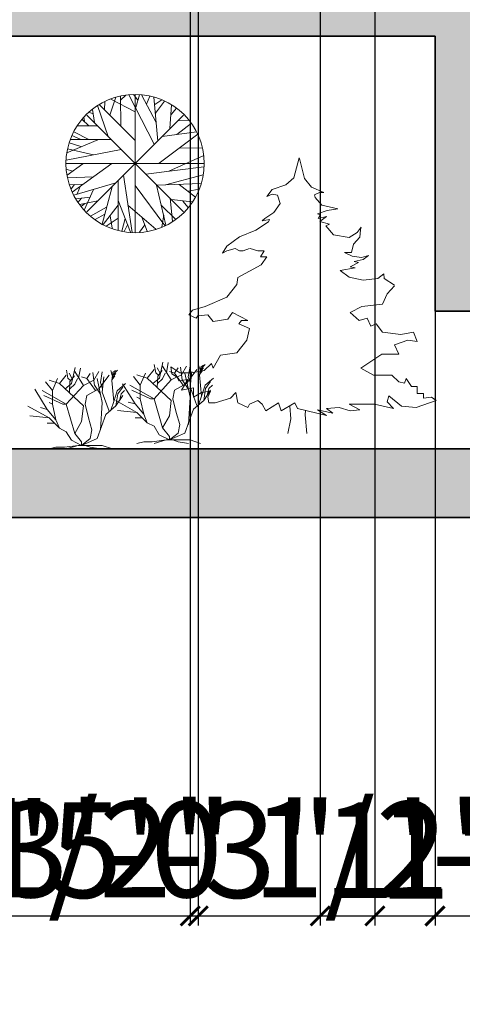
# Model space of a CAD drawing. Units: inches. Extents: x 1763 to 2368, y 1500 to 2097.
# Tile 2 of 24: x 1936 to 1994, y 1500 to 1628. Entities that reach past the tile are written whole.
import ezdxf

# ---------------------------------------------------------------- set-up
doc = ezdxf.new("R2010")
doc.units = ezdxf.units.IN
for name, color, linetype, lineweight in [('A-ANNO-DIMS', 2, 'Continuous', 18), ('A-WALL', 7, 'Continuous', 35), ('A-WALL-PATT', 7, 'Continuous', 13), ('trees', 3, 'Continuous', 13)]:
    doc.layers.add(name, color=color, linetype=linetype, lineweight=lineweight)
doc.styles.get("Standard").update_dxf_attribs({"font": 'arial.ttf'})
doc.dimstyles.new('ISO-25', dxfattribs={"dimtxt": 12.5, "dimasz": 2.5, "dimexe": 1.25, "dimexo": 0.625, "dimtad": 1, "dimdec": 0, "dimlunit": 4, "dimtxsty": 'Standard', "dimblk": 'ARCHTICK', "dimcen": 2.5, "dimclrd": 3, "dimclrt": 4, "dimadec": 0, "dimazin": 0, "dimtfac": 1, "dimtdec": 0, "dimtmove": 0, "dimatfit": 3, "dimfxl": 1, "dimarcsym": 0})

# ---------------------------------------------------------------- blocks, each defined once
blk = doc.blocks.new('*U7')
for p, q in [((-8.263, 7.598), (-8.747, 14.105)), ((-0.771, 9.56), (-0.69, 11.833)), ((-9.75, 0), (-8.263, 7.598)), ((0, 0), (-0.771, 9.56))]:
    blk.add_line(p, q)
for points in [[(-3.9, 142.35), (-6.596, 132.037), (-10.801, 128.443), (-17.81, 126.047), (-20.614, 122.452), (-17.81, 123.65), (-15.007, 123.051), (-13.605, 118.858), (-16.876, 114.065), (-21.549, 111.07), (-22.951, 109.872), (-19.212, 110.471), (-19.68, 109.273), (-26.222, 105.079), (-34.633, 101.485), (-41.175, 96.693), (-43.511, 93.098), (-41.175, 94.296), (-36.969, 95.494), (-34.633, 94.296), (-32.764, 94.296), (-29.493, 95.494)], [(-3.759, 141.97), (-1.074, 131.643), (2.437, 127.141), (8.84, 124.493), (6.568, 124.493), (4.09, 123.169), (4.296, 121.846), (7.807, 117.874), (16.069, 116.02), (10.492, 115.226), (5.535, 113.372), (6.981, 112.843), (5.948, 110.989), (10.286, 112.048), (6.775, 109.401), (11.732, 108.077), (9.873, 107.282), (13.797, 102.516), (21.852, 101.192), (25.983, 103.84), (28.048, 106.488), (27.842, 105.164), (27.429, 101.457), (24.124, 97.75), (23.091, 93.513), (19.58, 93.513), (23.505, 91.66), (28.255, 90.866), (31.973, 91.925), (29.081, 89.806), (24.537, 88.747), (26.809, 88.218), (22.472, 86.099), (24.95, 85.57), (17.308, 84.246), (21.852, 80.804), (29.081, 79.215), (36.723, 80.009), (39.821, 82.392), (40.028, 80.009), (45.398, 76.567)], [(-29.25, 95.55), (-25.287, 94.296), (-22.016, 94.296), (-23.885, 91.301), (-20.614, 91.301), (-23.418, 87.108), (-35.567, 80.518), (-36.035, 76.924), (-41.175, 70.334), (-52.389, 65.542), (-58.931, 63.744), (-60.8, 61.348), (-57.062, 59.551), (-56.128, 60.749), (-50.987, 61.348), (-48.184, 57.754), (-40.707, 58.952), (-38.371, 62.546), (-30.427, 58.353), (-33.698, 58.353), (-35.1, 56.556), (-29.493, 54.159), (-30.894, 48.169), (-36.035, 41.579), (-44.446, 40.381), (-48.184, 33.791), (-49.118, 36.188), (-52.857, 32.593), (-59.399, 31.395), (-65.473, 31.395), (-70.146, 34.39), (-69.679, 30.796), (-66.875, 28.999), (-65.941, 27.202), (-61.268, 27.801), (-64.539, 22.409), (-58.464, 23.607), (-58.464, 18.815), (-54.258, 21.211), (-49.586, 21.81), (-50.987, 18.815), (-50.52, 15.82), (-47.249, 15.82), (-39.306, 18.216), (-36.502, 21.211), (-35.567, 15.82), (-30.427, 13.423), (-29.493, 15.221), (-25.287, 17.018), (-22.951, 15.221), (-21.081, 11.626), (-14.539, 15.82), (-13.138, 11.626), (-6.128, 15.82), (-4.726, 12.824), (10.226, 9.23), (5.554, 12.225), (13.497, 10.428), (10.226, 12.824), (16.768, 13.423), (22.376, 11.626), (27.516, 12.225), (21.909, 15.221), (34.993, 15.221), (44.806, 12.824), (41.535, 16.419), (42.469, 19.414), (49.011, 14.023), (56.487, 13.423), (66.768, 17.018), (64.431, 18.815), (60.226, 18.216), (60.226, 20.612), (56.955, 20.612), (56.955, 24.206), (54.151, 24.206), (51.348, 28.4), (50.413, 26.004), (47.609, 26.603), (43.871, 30.197), (38.731, 30.197), (34.525, 30.197), (27.983, 33.791), (38.731, 40.98), (47.609, 40.98), (45.273, 45.773), (52.282, 48.169), (56.955, 47.57), (55.086, 52.362), (48.544, 51.164), (39.198, 52.362), (35.927, 56.556), (33.123, 55.357), (31.254, 59.551), (27.049, 58.353), (22.376, 62.546), (28.451, 65.542), (39.198, 66.74), (41.535, 72.131), (45.273, 76.325)]]:
    blk.add_lwpolyline(points)
blk = doc.blocks.new('*U16')
for p, q in [((2.426, 54.9406), (-1.4472, 59.9056)), ((0, 59.9996), (0, -60)), ((-26.4472, 46.5894), (-26.2712, 53.8116)), ((-22.0458, 42.0753), (-16.5881, 57.6486)), ((-21.1656, 55.8436), (-0.0388, 45.0094)), ((-12.5388, 54.9406), (-7.9613, 59.4546)), ((-12.3627, 32.1443), (-12.5388, 58.7776)), ((-5.3205, 59.6806), (16.5105, 16.7963)), ((0.4894, 48.6208), (3.6584, 59.6806)), ((18.2711, 35.5298), (5.419, 59.6806)), ((9.8203, 51.5549), (12.8133, 58.5516)), ((19.6795, 19.5047), (16.3344, 57.6486)), ((17.0387, 51.1035), (23.2006, 55.1666)), ((17.7429, 43.6552), (25.4894, 54.2636)), ((-40.1797, 44.558), (-36.4825, 43.2038)), ((-37.0107, 47.0408), (-35.25, 35.5298)), ((-32.6092, 50.4264), (-23.2782, 23.5674)), ((-31.2008, 51.1035), (-0.2149, 20.1818)), ((31.6513, 50.8778), (30.2429, 30.5643)), ((31.1232, 42.5267), (35.8767, 48.1693)), ((-45.8134, 38.2383), (-40.5318, 33.0471)), ((-43.8768, 36.4326), (-44.405, 40.2696)), ((42, 42), (-42, -42)), ((42, -42), (-42, 42)), ((36.2288, 25.1474), (48.9049, 35.0784)), ((37.1091, 37.1098), (46.6161, 37.5612)), ((-53.2078, 27.4044), (-40.1797, 20.859)), ((-49.8627, 32.8214), (-32.7853, 32.8214)), ((23.3767, 23.3417), (53.3063, 27.4044)), ((-32.2571, 20.6333), (-59.1937, 9.348)), ((-57.081, 17.9248), (-47.0458, 14.7649)), ((-56.0247, 20.859), (-20.8134, 20.859)), ((-54.7923, 24.4702), (-47.75, 21.0847)), ((54.3626, 25.3731), (20.9119, 0.3198)), ((-59.7219, 2.8025), (-12.0106, 12.0565)), ((-58.6656, 12.7336), (-35.9543, 7.5424)), ((38.5175, 13.4107), (58.2359, 13.6364)), ((-54.6162, -24.7335), (-20.2853, 0.0941)), ((29.3626, -6.6771), (59.4682, 7.091)), ((-60, 0), (60, 0)), ((-59.7219, -4.8714), (-54.2641, -6.6771)), ((-45.2853, -0.1316), (-59.0177, -10.0627)), ((9.2922, -9.1598), (59.6443, -2.8401)), ((-58.4895, -12.3197), (-36.4825, -11.6426)), ((-53.2078, -27.442), (-16.7641, -16.6081)), ((-14.8275, -15.0282), (-14.6515, -57.6865)), ((-10.074, -10.0627), (-2.5036, -59.7178)), ((26.3697, -18.4138), (58.9401, -9.8369)), ((-57.081, -18.4138), (-45.2853, -17.9624)), ((-52.6797, -18.188), (-55.4966, -22.0251)), ((-47.2219, -19.3166), (-50.2148, -26.3135)), ((-35.9543, -22.4765), (-44.0529, -40.5329)), ((-19.9331, -20.2194), (-28.5599, -52.721)), ((-0.0388, -19.0909), (25.8415, -53.8495)), ((18.6232, -18.6394), (26.7218, -53.3981)), ((18.7992, -18.6394), (57.3556, -17.2853)), ((38.1654, -18.188), (52.426, -29.0219)), ((45.9119, -24.0564), (55.595, -22.2508)), ((-38.9472, -29.0219), (-51.4472, -30.6018)), ((-46.5177, -30.1504), (-49.5106, -33.536)), ((-32.4331, -32.4075), (-48.1021, -35.5674)), ((-14.6515, -32.1818), (-3.912, -59.4922)), ((30.419, -30.1504), (32.3556, -50.0125)), ((31.4753, -31.279), (49.6091, -33.3103)), ((41.5105, -32.6332), (46.088, -38.0501)), ((-43.7008, -34.6645), (-46.6937, -37.373)), ((-24.6867, -37.8244), (-38.7712, -45.7241)), ((-14.6515, -36.2445), (-27.6797, -52.9467)), ((-6.2008, -36.2445), (17.919, -57.0094)), ((22.8485, -36.4702), (35.3485, -48.4326)), ((-26.2712, -43.9185), (-34.7219, -48.6583)), ((-14.6515, -47.3041), (-25.0388, -54.3009)), ((-21.5177, -45.4984), (-19.9331, -56.1065)), ((-8.4895, -47.5298), (-11.4825, -58.5893)), ((5.9471, -46.6269), (10.5246, -58.5893)), ((24.7852, -44.8213), (23.0246, -54.978)), ((-6.3768, -52.721), (-9.3698, -58.815)), ((8.4119, -53.1724), (3.8344, -59.4922))]:
    blk.add_line(p, q)
blk.add_circle((0, 0), 60)
blk = doc.blocks.new('*U17')
for p, q in [((-12.471, 19.775), (-12.898, 22.044)), ((-11.433, 18.289), (-10.457, 22.749)), ((-9.48, 19.775), (-8.992, 22.592)), ((0.041, 20.714), (1.384, 22.044)), ((-16.8, 16.32), (-15.36, 19.68)), ((-14.88, 18.24), (-12.96, 20.64)), ((-11.677, 19.071), (-12.471, 19.775)), ((-11.28, 19.619), (-12.104, 21.184)), ((-11.921, 18.836), (-10.64, 20.401)), ((-10.579, 18.054), (-9.846, 19.697)), ((-8.16, 17.76), (-10.56, 21.6)), ((-7.2, 19.68), (-8.64, 20.16)), ((-7.2, 19.68), (-6.24, 21.12)), ((-4.8, 16.32), (-7.2, 19.68)), ((-5.086, 17.741), (-5.513, 21.34)), ((-5.28, 19.2), (-3.84, 21.6)), ((-2.88, 12.96), (-4.32, 19.68)), ((-3.84, 16.8), (-0.96, 20.64)), ((-3.377, 18.602), (-2.888, 21.575)), ((-2.88, 15.84), (-2.4, 20.16)), ((-0.508, 21.888), (-0.081, 20.558)), ((-0.203, 19.149), (0.102, 21.34)), ((-0.142, 19.384), (0.59, 20.401)), ((-0.02, 20.01), (0.896, 21.105)), ((0.102, 21.34), (0.835, 21.888)), ((-18.24, 11.04), (-21.755, 16.655)), ((-16.8, 16.32), (-18.72, 18.72)), ((-14.88, 18.24), (-17.76, 19.2)), ((-8.16, 12), (-14.88, 18.24)), ((-13.325, 16.724), (-11.433, 18.289)), ((-12.96, 12.48), (-8.16, 17.76)), ((-12.043, 15.628), (-11.921, 18.836)), ((-11.982, 16.802), (-10.579, 18.054)), ((-8.16, 17.76), (-5.28, 19.2)), ((-7.2, 14.88), (-3.84, 16.8)), ((-3.377, 15.315), (-5.086, 17.819)), ((-2.766, 16.802), (-3.377, 18.602)), ((0.346, 13.203), (-0.203, 19.149)), ((1.323, 16.254), (3.642, 18.289)), ((1.44, 15.36), (2.88, 17.28)), ((-12.96, 12.48), (-19.68, 16.32)), ((-13.92, 12.48), (-19.2, 14.88)), ((-16.8, 12.48), (-16.8, 16.32)), ((-7.68, 12.48), (-7.2, 14.88)), ((-0.96, 10.56), (-2.88, 15.84)), ((0.346, 13.203), (1.323, 16.254)), ((0.96, 12), (1.44, 15.36)), ((0.96, 12), (2.88, 14.88)), ((1.92, 13.44), (2.4, 15.36)), ((2.4, 15.36), (3.36, 16.32)), ((-17.76, 8.64), (-23.663, 11.961)), ((-18.24, 11.04), (-20.16, 11.52)), ((-15.84, 8.16), (-18.24, 11.04)), ((-16.8, 12.48), (-17.76, 12.96)), ((-15.84, 8.16), (-16.8, 12.48)), ((-12.96, 12.48), (-13.92, 12.48)), ((-10.56, 4.32), (-12.96, 12.48)), ((-8.64, 7.68), (-8.16, 12)), ((-6.72, 8.64), (-7.68, 12.48)), ((-3.36, 5.28), (-2.88, 12.96)), ((-1.92, 9.6), (0.96, 12)), ((-0.48, 10.8), (0.346, 13.203)), ((-17.76, 8.64), (-23.128, 9.222)), ((-14.88, 5.76), (-17.76, 8.64)), ((-5.76, 5.28), (-6.72, 8.64)), ((-4.32, 2.88), (-1.92, 9.6)), ((-16.32, 7.2), (-18.24, 7.2)), ((-14.88, 5.76), (-15.84, 8.16)), ((-12.96, 4.8), (-14.88, 5.76)), ((-10.56, 4.32), (-8.64, 7.68)), ((-11.52, 2.4), (-12.96, 4.8)), ((-8.64, 1.92), (-10.56, 4.32)), ((-8.64, 0.96), (-4.32, 2.88)), ((-8.64, 0.96), (-6.24, 2.88)), ((-6.24, 2.88), (-5.76, 5.28)), ((-15.84, 0.48), (-17.76, 0)), ((-13.44, 0.48), (-15.84, 0.48)), ((-9.6, 0.96), (-13.44, 0.48)), ((-9.6, 0.96), (-12.96, 0)), ((-8.64, 0.96), (-11.52, 2.4)), ((-9.6, 0.96), (-7.68, 0.96)), ((-8.64, 0.96), (-8.64, 1.92)), ((-8.64, 0.96), (-2.88, 0.96)), ((-7.68, 0.96), (-6.24, 0.48)), ((-6.24, 0.48), (-3.36, 0)), ((-2.88, 0.96), (0, 0))]:
    blk.add_line(p, q)
blk = doc.blocks.new('_ArchTick')
at = {"color": 0, "linetype": 'ByBlock', "const_width": 0.15}
blk.add_lwpolyline([(-0.5, -0.5), (0.5, 0.5)], dxfattribs=at)
blk = doc.blocks.new('*D39')
at = {"layer": 'A-ANNO-DIMS', "color": 0, "lineweight": -2, "transparency": 16777216}
for p, q in [((1829.09, 1562.65), (1829.09, 1509.91)), ((2003.86, 1562.65), (2003.86, 1509.91))]:
    blk.add_line(p, q, dxfattribs=at)
at = {"layer": 'A-ANNO-DIMS', "color": 3, "lineweight": -2, "transparency": 16777216}
blk.add_line((1829.09, 1511.16), (2003.86, 1511.16), dxfattribs=at)
at = {"layer": 'Defpoints', "color": 0, "transparency": 16777216}
for p in [(1829.09, 1563.27), (2003.86, 1563.27), (2003.86, 1511.16)]:
    blk.add_point(p, dxfattribs=at)
at = {"layer": 'A-ANNO-DIMS', "color": 3, "lineweight": -2, "transparency": 16777216, "xscale": 2.5, "yscale": 2.5, "zscale": 2.5, "rotation": 180}
blk.add_blockref('_ArchTick', (1829.09, 1511.16), dxfattribs=at)
at = {"layer": 'A-ANNO-DIMS', "color": 3, "lineweight": -2, "transparency": 16777216, "xscale": 2.5, "yscale": 2.5, "zscale": 2.5}
blk.add_blockref('_ArchTick', (2003.86, 1511.16), dxfattribs=at)
at = {"layer": 'A-ANNO-DIMS', "color": 4, "transparency": 16777216, "insert": (1916.48, 1518.06), "char_height": 12.5, "attachment_point": 5}
blk.add_mtext('14\'-7"', dxfattribs=at)
blk = doc.blocks.new('*D57')
at = {"layer": 'A-ANNO-DIMS', "color": 0, "lineweight": -2, "transparency": 16777216}
for p, q in [((1927.07, 1625.65), (1927.07, 1509.91)), ((1990.09, 1625.65), (1990.09, 1509.91))]:
    blk.add_line(p, q, dxfattribs=at)
at = {"layer": 'A-ANNO-DIMS', "color": 3, "lineweight": -2, "transparency": 16777216}
blk.add_line((1927.07, 1511.16), (1990.09, 1511.16), dxfattribs=at)
at = {"layer": 'Defpoints', "color": 0, "transparency": 16777216}
for p in [(1927.07, 1626.27), (1990.09, 1626.27), (1990.09, 1511.16)]:
    blk.add_point(p, dxfattribs=at)
at = {"layer": 'A-ANNO-DIMS', "color": 3, "lineweight": -2, "transparency": 16777216, "xscale": 2.5, "yscale": 2.5, "zscale": 2.5, "rotation": 180}
blk.add_blockref('_ArchTick', (1927.07, 1511.16), dxfattribs=at)
at = {"layer": 'A-ANNO-DIMS', "color": 3, "lineweight": -2, "transparency": 16777216, "xscale": 2.5, "yscale": 2.5, "zscale": 2.5}
blk.add_blockref('_ArchTick', (1990.09, 1511.16), dxfattribs=at)
at = {"layer": 'A-ANNO-DIMS', "color": 4, "transparency": 16777216, "insert": (1958.58, 1518.17), "char_height": 12.5, "attachment_point": 5}
blk.add_mtext('5\'-3"', dxfattribs=at)
blk = doc.blocks.new('*D68')
at = {"layer": 'A-ANNO-DIMS', "color": 0, "lineweight": -2, "transparency": 16777216}
for p, q in [((1895.59, 1879.65), (1895.59, 1509.91)), ((1932.01, 1879.65), (1932.01, 1509.91))]:
    blk.add_line(p, q, dxfattribs=at)
at = {"layer": 'A-ANNO-DIMS', "color": 3, "lineweight": -2, "transparency": 16777216}
for p, q in [((1895.59, 1511.16), (1932.01, 1511.16)), ((1932.01, 1511.16), (1998.11, 1511.16))]:
    blk.add_line(p, q, dxfattribs=at)
at = {"layer": 'Defpoints', "color": 0, "transparency": 16777216}
for p in [(1895.59, 1880.27), (1932.01, 1880.27), (1932.01, 1511.16)]:
    blk.add_point(p, dxfattribs=at)
at = {"layer": 'A-ANNO-DIMS', "color": 3, "lineweight": -2, "transparency": 16777216, "xscale": 2.5, "yscale": 2.5, "zscale": 2.5, "rotation": 180}
blk.add_blockref('_ArchTick', (1895.59, 1511.16), dxfattribs=at)
at = {"layer": 'A-ANNO-DIMS', "color": 3, "lineweight": -2, "transparency": 16777216, "xscale": 2.5, "yscale": 2.5, "zscale": 2.5}
blk.add_blockref('_ArchTick', (1932.01, 1511.16), dxfattribs=at)
at = {"layer": 'A-ANNO-DIMS', "color": 4, "transparency": 16777216, "insert": (1966.31, 1518.25), "char_height": 12.5, "attachment_point": 5}
blk.add_mtext('3\'-0 1/2"', dxfattribs=at)
blk = doc.blocks.new('*D69')
at = {"layer": 'A-ANNO-DIMS', "color": 0, "lineweight": -2, "transparency": 16777216}
for p, q in [((1838.09, 1879.65), (1838.09, 1509.91)), ((1895.59, 1879.65), (1895.59, 1509.91))]:
    blk.add_line(p, q, dxfattribs=at)
at = {"layer": 'A-ANNO-DIMS', "color": 3, "lineweight": -2, "transparency": 16777216}
for p, q in [((1838.09, 1511.16), (1895.59, 1511.16)), ((1895.59, 1511.16), (1962.2, 1511.16))]:
    blk.add_line(p, q, dxfattribs=at)
at = {"layer": 'Defpoints', "color": 0, "transparency": 16777216}
for p in [(1838.09, 1880.27), (1895.59, 1880.27), (1895.59, 1511.16)]:
    blk.add_point(p, dxfattribs=at)
at = {"layer": 'A-ANNO-DIMS', "color": 3, "lineweight": -2, "transparency": 16777216, "xscale": 2.5, "yscale": 2.5, "zscale": 2.5, "rotation": 180}
blk.add_blockref('_ArchTick', (1838.09, 1511.16), dxfattribs=at)
at = {"layer": 'A-ANNO-DIMS', "color": 3, "lineweight": -2, "transparency": 16777216, "xscale": 2.5, "yscale": 2.5, "zscale": 2.5}
blk.add_blockref('_ArchTick', (1895.59, 1511.16), dxfattribs=at)
at = {"layer": 'A-ANNO-DIMS', "color": 4, "transparency": 16777216, "insert": (1930.15, 1518.24), "char_height": 12.5, "attachment_point": 5}
blk.add_mtext('4\'-9 1/2"', dxfattribs=at)
blk = doc.blocks.new('*D70')
at = {"layer": 'A-ANNO-DIMS', "color": 0, "lineweight": -2, "transparency": 16777216}
for p, q in [((1959.13, 1879.65), (1959.13, 1509.91)), ((1982.23, 1879.65), (1982.23, 1509.91))]:
    blk.add_line(p, q, dxfattribs=at)
at = {"layer": 'A-ANNO-DIMS', "color": 3, "lineweight": -2, "transparency": 16777216}
for p, q in [((1959.13, 1511.16), (1982.23, 1511.16)), ((1982.23, 1511.16), (2027.75, 1511.16))]:
    blk.add_line(p, q, dxfattribs=at)
at = {"layer": 'Defpoints', "color": 0, "transparency": 16777216}
for p in [(1959.13, 1880.27), (1982.23, 1880.27), (1982.23, 1511.16)]:
    blk.add_point(p, dxfattribs=at)
at = {"layer": 'A-ANNO-DIMS', "color": 3, "lineweight": -2, "transparency": 16777216, "xscale": 2.5, "yscale": 2.5, "zscale": 2.5, "rotation": 180}
blk.add_blockref('_ArchTick', (1959.13, 1511.16), dxfattribs=at)
at = {"layer": 'A-ANNO-DIMS', "color": 3, "lineweight": -2, "transparency": 16777216, "xscale": 2.5, "yscale": 2.5, "zscale": 2.5}
blk.add_blockref('_ArchTick', (1982.23, 1511.16), dxfattribs=at)
at = {"layer": 'A-ANNO-DIMS', "color": 4, "transparency": 16777216, "insert": (2006.24, 1518.06), "char_height": 12.5, "attachment_point": 5}
blk.add_mtext('1\'-11"', dxfattribs=at)
blk = doc.blocks.new('*D77')
at = {"layer": 'A-ANNO-DIMS', "color": 0, "lineweight": -2, "transparency": 16777216}
for p, q in [((1975.09, 1972.65), (1975.09, 1509.91)), ((1996.09, 1972.65), (1996.09, 1509.91))]:
    blk.add_line(p, q, dxfattribs=at)
at = {"layer": 'A-ANNO-DIMS', "color": 3, "lineweight": -2, "transparency": 16777216}
for p, q in [((1975.09, 1511.16), (1996.09, 1511.16)), ((1996.09, 1511.16), (2031.89, 1511.16))]:
    blk.add_line(p, q, dxfattribs=at)
at = {"layer": 'Defpoints', "color": 0, "transparency": 16777216}
for p in [(1975.09, 1973.27), (1996.09, 1973.27), (1996.09, 1511.16)]:
    blk.add_point(p, dxfattribs=at)
at = {"layer": 'A-ANNO-DIMS', "color": 3, "lineweight": -2, "transparency": 16777216, "xscale": 2.5, "yscale": 2.5, "zscale": 2.5, "rotation": 180}
blk.add_blockref('_ArchTick', (1975.09, 1511.16), dxfattribs=at)
at = {"layer": 'A-ANNO-DIMS', "color": 3, "lineweight": -2, "transparency": 16777216, "xscale": 2.5, "yscale": 2.5, "zscale": 2.5}
blk.add_blockref('_ArchTick', (1996.09, 1511.16), dxfattribs=at)
at = {"layer": 'A-ANNO-DIMS', "color": 4, "transparency": 16777216, "insert": (2015.24, 1518.16), "char_height": 12.5, "attachment_point": 5}
blk.add_mtext('1\'-9"', dxfattribs=at)
blk = doc.blocks.new('*D87')
at = {"layer": 'A-ANNO-DIMS', "color": 0, "lineweight": -2, "transparency": 16777216}
for p, q in [((1958.09, 1980.65), (1958.09, 1509.91)), ((1975.09, 1980.65), (1975.09, 1509.91))]:
    blk.add_line(p, q, dxfattribs=at)
at = {"layer": 'A-ANNO-DIMS', "color": 3, "lineweight": -2, "transparency": 16777216}
for p, q in [((1958.09, 1511.16), (1975.09, 1511.16)), ((1975.09, 1511.16), (2010.89, 1511.16))]:
    blk.add_line(p, q, dxfattribs=at)
at = {"layer": 'Defpoints', "color": 0, "transparency": 16777216}
for p in [(1958.09, 1981.27), (1975.09, 1981.27), (1975.09, 1511.16)]:
    blk.add_point(p, dxfattribs=at)
at = {"layer": 'A-ANNO-DIMS', "color": 3, "lineweight": -2, "transparency": 16777216, "xscale": 2.5, "yscale": 2.5, "zscale": 2.5, "rotation": 180}
blk.add_blockref('_ArchTick', (1958.09, 1511.16), dxfattribs=at)
at = {"layer": 'A-ANNO-DIMS', "color": 3, "lineweight": -2, "transparency": 16777216, "xscale": 2.5, "yscale": 2.5, "zscale": 2.5}
blk.add_blockref('_ArchTick', (1975.09, 1511.16), dxfattribs=at)
at = {"layer": 'A-ANNO-DIMS', "color": 4, "transparency": 16777216, "insert": (1994.24, 1518.16), "char_height": 12.5, "attachment_point": 5}
blk.add_mtext('1\'-5"', dxfattribs=at)

msp = doc.modelspace()

# ---------------------------------------------------------------- hatches: boundary and pattern name
at = {"layer": 'A-WALL-PATT'}
h = msp.add_hatch(color=256, dxfattribs=at)
h.dxf.hatch_style = 1
h.paths.add_polyline_path([(1838.09, 2034.27), (1838.09, 2043.27), (1829.09, 2043.27), (1829.09, 1953.39), (1838.09, 1953.39)])
h.paths.add_polyline_path([(1838.09, 1913.1), (1829.09, 1913.1), (1829.09, 1862.2), (1838.09, 1862.2)])
h.paths.add_polyline_path([(1838.09, 1825.59), (1829.09, 1825.59), (1829.09, 1738.64), (1838.09, 1738.64)])
h.paths.add_polyline_path([(1895.59, 1885.27), (1838.09, 1885.27), (1838.09, 1880.27), (1895.59, 1880.27)])
h.paths.add_polyline_path([(1857.39, 1784.27), (1838.09, 1784.27), (1838.09, 1779.27), (1857.39, 1779.27)])
h.paths.add_polyline_path([(1958.09, 1981.27), (1971.46, 1981.27), (1971.46, 1986.27), (1968.57, 1986.27), (1958.09, 1986.27), (1953.09, 1986.27), (1927.39, 1986.27), (1927.39, 1981.27), (1953.09, 1981.27), (1953.09, 1885.27), (1932.01, 1885.27), (1932.01, 1880.27), (1959.13, 1880.27), (1959.13, 1883.74), (1959.13, 1885.27), (1958.09, 1885.27)])
h.paths.add_polyline_path([(2018.09, 1981.27), (2031.02, 1981.27), (2031.02, 1986.27), (2018.09, 1986.27), (2013.09, 1986.27), (2001.23, 1986.27), (2001.23, 1981.27), (2013.09, 1981.27), (2013.09, 1885.27), (1982.18, 1885.27, -0.016629), (1982.23, 1883.74), (1982.23, 1880.27), (2049.69, 1880.27), (2049.69, 1883.74, -0.016629), (2049.74, 1885.27), (2018.09, 1885.27)])
h.paths.add_polyline_path([(2083.09, 1981.27), (2120.61, 1981.27), (2120.61, 1986.27), (2083.09, 1986.27), (2078.09, 1986.27), (2063.14, 1986.27), (2063.14, 1981.27), (2078.09, 1981.27), (2078.09, 1885.27), (2072.78, 1885.27), (2072.78, 1883.74), (2072.78, 1880.27), (2078.09, 1880.27), (2078.09, 1866.87), (2081.56, 1866.87, -0.016629), (2083.09, 1866.82)])
h.paths.add_polyline_path([(1871.68, 1635.27), (1838.09, 1635.27), (1838.09, 1626.27), (1871.68, 1626.27)], flags=17)
h.paths.add_polyline_path([(2100.58, 1688.27), (2060.09, 1688.27), (2060.09, 1679.27), (2100.58, 1679.27)], flags=17)
h.paths.add_polyline_path([(2180.09, 1688.27), (2148.74, 1688.27), (2148.74, 1679.27), (2180.09, 1679.27)], flags=17)
h.paths.add_polyline_path([(2189.09, 1746.22), (2180.09, 1746.22), (2180.09, 1743.42), (2180.12, 1743.42), (2180.12, 1726.72), (2180.09, 1572.27), (2034.91, 1572.27), (2034.91, 1565.6), (2034.91, 1563.27), (2189.09, 1563.27)])
h.paths.add_polyline_path([(2060.09, 1802.35, -0.016629), (2058.56, 1802.3), (2055.09, 1802.3), (2055.09, 1635.27), (2042.48, 1635.27), (2042.48, 1629.74), (2042.48, 1626.27), (2055.09, 1626.27), (2055.09, 1599.27), (2040.27, 1599.27), (2040.27, 1590.27), (2060.09, 1590.27)])
h.paths.add_polyline_path([(2019.39, 1629.74, -0.060569), (2020.06, 1635.27), (1995.09, 1635.27), (1990.09, 1635.27), (1927.07, 1635.27), (1927.07, 1626.27), (1990.09, 1626.27), (1990.09, 1590.27), (1995.09, 1590.27), (2005.2, 1590.27), (2005.2, 1599.27), (1995.09, 1599.27), (1995.09, 1626.27), (2019.39, 1626.27)])
edge = h.paths.add_edge_path()
edge.add_line((2180.09, 1837.27), (2167.2, 1837.27))
edge.add_spline(control_points=[(2167.2, 1837.27), (2167.19, 1837.27), (2167.18, 1837.27), (2167.18, 1837.27)], knot_values=[168.955493, 168.955493, 168.955493, 168.955493, 169.065871, 169.065871, 169.065871, 169.065871], degree=3, periodic=0)
edge.add_spline(control_points=[(2167.18, 1837.27), (2166.56, 1837.38), (2166.33, 1846.16), (2165.71, 1846.24)], knot_values=[159.864705, 159.864705, 159.864705, 159.864705, 168.955493, 168.955493, 168.955493, 168.955493], degree=3, periodic=0)
edge.add_line((2167.12, 1837.27), (2163.16, 1837.27))
edge.add_spline(control_points=[(2163.16, 1837.27), (2163.16, 1837.27), (2163.16, 1837.27), (2163.15, 1837.27)], knot_values=[150.537172, 150.537172, 150.537172, 150.537172, 150.553797, 150.553797, 150.553797, 150.553797], degree=3, periodic=0)
edge.add_spline(control_points=[(2163.15, 1837.27), (2162.29, 1837.29), (2161.59, 1846.23), (2160.88, 1846.24)], knot_values=[141.293426, 141.293426, 141.293426, 141.293426, 150.537172, 150.537172, 150.537172, 150.537172], degree=3, periodic=0)
edge.add_line((2163.08, 1837.27), (2158.7, 1837.27))
edge.add_spline(control_points=[(2158.7, 1837.27), (2158.7, 1837.27), (2158.7, 1837.27), (2158.7, 1837.27)], knot_values=[132.033544, 132.033544, 132.033544, 132.033544, 132.049151, 132.049151, 132.049151, 132.049151], degree=3, periodic=0)
edge.add_spline(control_points=[(2158.7, 1837.27), (2157.97, 1837.29), (2157.26, 1846.23), (2156.39, 1846.24)], knot_values=[122.786021, 122.786021, 122.786021, 122.786021, 132.033544, 132.033544, 132.033544, 132.033544], degree=3, periodic=0)
edge.add_line((2158.63, 1837.27), (2153.84, 1837.27))
edge.add_spline(control_points=[(2153.84, 1837.27), (2153.83, 1837.27), (2153.82, 1837.27), (2153.82, 1837.27)], knot_values=[113.451585, 113.451585, 113.451585, 113.451585, 113.562103, 113.562103, 113.562103, 113.562103], degree=3, periodic=0)
edge.add_spline(control_points=[(2153.82, 1837.27), (2153.17, 1837.38), (2152.88, 1846.19), (2152.4, 1846.24)], knot_values=[0, 0, 0, 0, 9.081854, 9.081854, 9.081854, 9.081854], degree=3, periodic=0)
edge.add_line((2153.76, 1837.27), (2150.39, 1837.27))
edge.add_spline(control_points=[(2150.39, 1837.27), (2150.38, 1837.27), (2150.37, 1837.27), (2150.36, 1837.27)], knot_values=[95.069382, 95.069382, 95.069382, 95.069382, 95.17519, 95.17519, 95.17519, 95.17519], degree=3, periodic=0)
edge.add_spline(control_points=[(2150.36, 1837.27), (2149.49, 1837.37), (2148.42, 1846.19), (2147.59, 1846.24)], knot_values=[85.824599, 85.824599, 85.824599, 85.824599, 95.069382, 95.069382, 95.069382, 95.069382], degree=3, periodic=0)
edge.add_line((2150.29, 1837.27), (2145.43, 1837.27))
edge.add_spline(control_points=[(2145.43, 1837.27), (2145.43, 1837.27), (2145.42, 1837.27), (2145.42, 1837.27)], knot_values=[76.505559, 76.505559, 76.505559, 76.505559, 76.547811, 76.547811, 76.547811, 76.547811], degree=3, periodic=0)
edge.add_spline(control_points=[(2145.42, 1837.27), (2144.68, 1837.31), (2143.8, 1846.19), (2142.95, 1846.24)], knot_values=[67.23945, 67.23945, 67.23945, 67.23945, 76.505559, 76.505559, 76.505559, 76.505559], degree=3, periodic=0)
edge.add_line((2145.35, 1837.27), (2134.57, 1837.27))
edge.add_spline(control_points=[(2134.57, 1837.27), (2134.57, 1837.27), (2134.56, 1837.27), (2134.56, 1837.27)], knot_values=[39.001463, 39.001463, 39.001463, 39.001463, 39.045107, 39.045107, 39.045107, 39.045107], degree=3, periodic=0)
edge.add_spline(control_points=[(2134.56, 1837.27), (2133.87, 1837.31), (2133.4, 1845.85), (2132.33, 1846.24)], knot_values=[29.79778, 29.79778, 29.79778, 29.79778, 39.001463, 39.001463, 39.001463, 39.001463], degree=3, periodic=0)
edge.add_line((2134.5, 1837.27), (2128.08, 1837.27))
edge.add_spline(control_points=[(2128.08, 1837.27), (2128.03, 1837.26), (2127.98, 1837.26), (2127.93, 1837.27)], knot_values=[19.482067, 19.482067, 19.482067, 19.482067, 19.869396, 19.869396, 19.869396, 19.869396], degree=3, periodic=0)
edge.add_spline(control_points=[(2125.01, 1846.24), (2126.16, 1844.66), (2126.82, 1837.57), (2127.93, 1837.27)], knot_values=[10.389805, 10.389805, 10.389805, 10.389805, 19.482067, 19.482067, 19.482067, 19.482067], degree=3, periodic=0)
edge.add_line((2127.93, 1837.27), (2083.09, 1837.27))
edge.add_line((2083.09, 1837.27), (2083.09, 1843.77))
edge.add_line((2083.09, 1843.77), (2081.56, 1843.77))
edge.add_line((2081.56, 1843.77), (2078.09, 1843.77))
edge.add_line((2078.09, 1843.77), (2078.09, 1837.27))
edge.add_line((2078.09, 1837.27), (2055.09, 1837.27))
edge.add_line((2055.09, 1837.27), (2055.09, 1825.4))
edge.add_line((2055.09, 1825.4), (2058.56, 1825.4))
edge.add_line((2058.56, 1825.4), (2060.09, 1825.4))
edge.add_line((2060.09, 1825.4), (2060.09, 1832.27))
edge.add_line((2060.09, 1832.27), (2122.44, 1832.27))
edge.add_spline(control_points=[(2122.44, 1832.27), (2122.73, 1832.58), (2123.01, 1832.62), (2123.28, 1832.27)], knot_values=[5.972033, 5.972033, 5.972033, 5.972033, 8.057258, 8.057258, 8.057258, 8.057258], degree=3, periodic=0)
edge.add_line((2123.28, 1832.27), (2137.95, 1832.27))
edge.add_spline(control_points=[(2137.95, 1832.27), (2137.96, 1832.27), (2137.97, 1832.27), (2137.98, 1832.27)], knot_values=[53.926862, 53.926862, 53.926862, 53.926862, 54.030075, 54.030075, 54.030075, 54.030075], degree=3, periodic=0)
edge.add_spline(control_points=[(2139.72, 1825.02), (2139.28, 1825.06), (2138.67, 1832.18), (2137.98, 1832.27)], knot_values=[54.030075, 54.030075, 54.030075, 54.030075, 61.445194, 61.445194, 61.445194, 61.445194], degree=3, periodic=0)
edge.add_line((2138.05, 1832.27), (2140.96, 1832.27))
edge.add_spline(control_points=[(2140.96, 1832.27), (2140.97, 1832.27), (2140.98, 1832.27), (2140.99, 1832.27)], knot_values=[68.854182, 68.854182, 68.854182, 68.854182, 68.971237, 68.971237, 68.971237, 68.971237], degree=3, periodic=0)
edge.add_spline(control_points=[(2143.19, 1825.02), (2142.44, 1825.07), (2141.56, 1832.16), (2140.99, 1832.27)], knot_values=[68.971237, 68.971237, 68.971237, 68.971237, 76.444911, 76.444911, 76.444911, 76.444911], degree=3, periodic=0)
edge.add_line((2141.04, 1832.27), (2145.43, 1832.27))
edge.add_spline(control_points=[(2145.43, 1832.27), (2145.44, 1832.27), (2145.45, 1832.27), (2145.46, 1832.27)], knot_values=[84.039047, 84.039047, 84.039047, 84.039047, 84.124041, 84.124041, 84.124041, 84.124041], degree=3, periodic=0)
edge.add_spline(control_points=[(2148.11, 1825.02), (2147.34, 1825.02), (2146.3, 1832.19), (2145.46, 1832.27)], knot_values=[84.124041, 84.124041, 84.124041, 84.124041, 91.773891, 91.773891, 91.773891, 91.773891], degree=3, periodic=0)
edge.add_line((2145.54, 1832.27), (2150.39, 1832.27))
edge.add_spline(control_points=[(2150.39, 1832.27), (2150.42, 1832.28), (2150.45, 1832.28), (2150.47, 1832.27)], knot_values=[99.381577, 99.381577, 99.381577, 99.381577, 99.573457, 99.573457, 99.573457, 99.573457], degree=3, periodic=0)
edge.add_spline(control_points=[(2153.97, 1825.02), (2153.09, 1825.28), (2151.53, 1832.1), (2150.47, 1832.27)], knot_values=[99.573457, 99.573457, 99.573457, 99.573457, 107.218357, 107.218357, 107.218357, 107.218357], degree=3, periodic=0)
edge.add_line((2150.57, 1832.27), (2155.6, 1832.27))
edge.add_spline(control_points=[(2155.6, 1832.27), (2155.6, 1832.27), (2155.61, 1832.27), (2155.62, 1832.27)], knot_values=[114.933058, 114.933058, 114.933058, 114.933058, 115.013624, 115.013624, 115.013624, 115.013624], degree=3, periodic=0)
edge.add_spline(control_points=[(2158.28, 1825.02), (2157.4, 1825.07), (2156.25, 1832.2), (2155.62, 1832.27)], knot_values=[115.013624, 115.013624, 115.013624, 115.013624, 122.616269, 122.616269, 122.616269, 122.616269], degree=3, periodic=0)
edge.add_line((2155.68, 1832.27), (2165.19, 1832.27))
edge.add_spline(control_points=[(2165.19, 1832.27), (2165.2, 1832.27), (2165.2, 1832.27), (2165.2, 1832.27)], knot_values=[145.488477, 145.488477, 145.488477, 145.488477, 145.516379, 145.516379, 145.516379, 145.516379], degree=3, periodic=0)
edge.add_spline(control_points=[(2167.45, 1825.02), (2166.96, 1825.02), (2166.06, 1832.25), (2165.2, 1832.27)], knot_values=[145.516379, 145.516379, 145.516379, 145.516379, 153.105469, 153.105469, 153.105469, 153.105469], degree=3, periodic=0)
edge.add_line((2165.29, 1832.27), (2168.93, 1832.27))
edge.add_spline(control_points=[(2168.93, 1832.27), (2168.98, 1832.29), (2169.04, 1832.29), (2169.1, 1832.27)], knot_values=[160.517439, 160.517439, 160.517439, 160.517439, 160.939723, 160.939723, 160.939723, 160.939723], degree=3, periodic=0)
edge.add_spline(control_points=[(2171.09, 1828.64), (2170.35, 1830.37), (2169.62, 1832.09), (2169.1, 1832.27)], knot_values=[160.939723, 160.939723, 160.939723, 160.939723, 164.738835, 164.738835, 164.738835, 164.738835], degree=3, periodic=0)
edge.add_line((2169.1, 1832.27), (2180.09, 1832.27))
edge.add_line((2180.09, 1832.27), (2180.09, 1837.27))
h.paths.add_polyline_path([(2189.09, 1885.52), (2180.09, 1885.52), (2180.09, 1813.32), (2180.12, 1813.32), (2180.12, 1796.62), (2180.12, 1795.26), (2189.09, 1795.26)])
h.paths.add_polyline_path([(2180.09, 1986.27), (2166.28, 1986.27), (2166.28, 1981.27), (2180.09, 1981.27)])
h.paths.add_polyline_path([(2189.09, 2043.27), (2180.09, 2043.27), (2180.09, 2034.27), (2180.09, 1934.11), (2189.09, 1934.11)])
h.paths.add_polyline_path([(1838.09, 1681.59), (1829.09, 1681.59), (1829.09, 1563.27), (2003.86, 1563.27), (2003.86, 1565.6), (2003.86, 1572.27), (1838.09, 1572.27)])

# ---------------------------------------------------------------- linework, layer by layer
at = {"layer": 'A-WALL'}
for p, q in [((1838.09, 1626.27), (1990.09, 1626.27)), ((1990.09, 1626.27), (1990.09, 1590.27)), ((1995.09, 1590.27), (1990.09, 1590.27)), ((2004.54, 1572.27), (1838.09, 1572.27))]:
    msp.add_line(p, q, dxfattribs=at)
msp.add_lwpolyline([(2003.86, 1563.27), (1829.09, 1563.27), (1829.09, 2043.27), (2189.09, 2043.27), (2189.09, 1563.27), (2034.91, 1563.27)], dxfattribs=at)

# ---------------------------------------------------------------- block references
at = {"layer": 'trees'}
for name, p, xscale, yscale, zscale in [('*U16', (1950.88, 1609.59), 0.1507671210362717, 0.1507671210362717, 0.1507671210362717), ('*U7', (1973.31, 1574.28), 0.2532954982956893, 0.2532954982956893, 0.2532954982956893), ('*U17', (1959.41, 1572.98), 0.4676307550764569, 0.4676307550764569, 0.4676307550764569), ('*U17', (1947.93, 1572.27), 0.4676307550764569, 0.4676307550764569, 0.4676307550764569)]:
    msp.add_blockref(name, p, dxfattribs=dict(at, xscale=xscale, yscale=yscale, zscale=zscale))

# ---------------------------------------------------------------- dimensions: what is measured, and where the dimension line sits
at = {"layer": 'A-ANNO-DIMS'}
for base, p1, p2, picture, middle in [((1975.09, 1511.16), (1958.09, 1981.27), (1975.09, 1981.27), '*D87', (1994.24, 1518.16)), ((1996.09, 1511.16), (1975.09, 1973.27), (1996.09, 1973.27), '*D77', (2015.24, 1518.16)), ((1895.59, 1511.16), (1838.09, 1880.27), (1895.59, 1880.27), '*D69', (1930.15, 1518.24)), ((1932.01, 1511.16), (1895.59, 1880.27), (1932.01, 1880.27), '*D68', (1966.31, 1518.25)), ((1982.23, 1511.16), (1959.13, 1880.27), (1982.23, 1880.27), '*D70', (2006.24, 1518.06)), ((1990.09, 1511.16), (1927.07, 1626.27), (1990.09, 1626.27), '*D57', (1958.58, 1518.17)), ((2003.86, 1511.16), (1829.09, 1563.27), (2003.86, 1563.27), '*D39', (1916.48, 1518.06))]:
    dim = msp.add_linear_dim(base=base, p1=p1, p2=p2, dimstyle='ISO-25', override={"dimdec": 1, "dimlfac": 1, "dimrnd": 0, "dimzin": 1, "dimdsep": 46, "dimlunit": 4, "dimfrac": 2}, dxfattribs=at)
    dim.commit()
    dim.dimension.update_dxf_attribs({"geometry": picture, "text_midpoint": middle})

doc.saveas('drawing.dxf')
